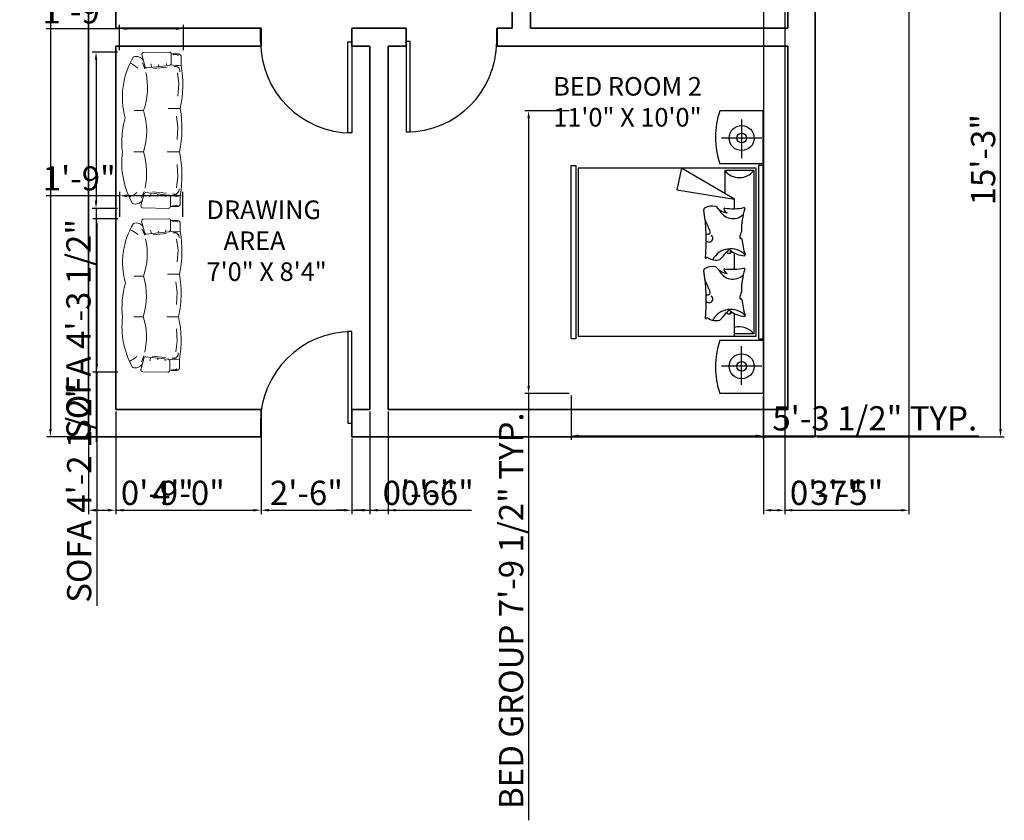
# Model space of a CAD drawing. Units: inches. Extents: x 3064 to 3427, y 2432 to 3115.
# Tile 1 of 3: x 3075 to 3401, y 2432 to 2696. Entities that reach past the tile are written whole.
import ezdxf

# ---------------------------------------------------------------- set-up
doc = ezdxf.new("R2010")
doc.units = ezdxf.units.IN
for name, color, linetype, lineweight in [('A-ANNO-DIMS', 2, 'Continuous', 13), ('A-AREA-IDEN', 7, 'Continuous', 18), ('A-DOOR', 4, 'Continuous', 25), ('A-WALL', 7, 'Continuous', 35), ('FUR', 42, 'Continuous', 18)]:
    doc.layers.add(name, color=color, linetype=linetype, lineweight=lineweight)
for name, color, linetype in [('HID', 11, 'Continuous'), ('SAN', 5, 'Continuous'), ('wood', 26, 'Continuous')]:
    doc.layers.add(name, color=color, linetype=linetype)
doc.styles.get("Standard").update_dxf_attribs({"font": 'arial.ttf'})
doc.dimstyles.new('ISO-25', dxfattribs={"dimtxt": 8, "dimasz": 2.5, "dimexe": 1.25, "dimexo": 0.625, "dimtad": 1, "dimdec": 0, "dimlunit": 4, "dimtxsty": 'Standard', "dimcen": 2.5, "dimadec": 0, "dimazin": 0, "dimtfac": 1, "dimtdec": 0, "dimtmove": 0, "dimatfit": 3, "dimfxl": 1, "dimarcsym": 0})

# ---------------------------------------------------------------- blocks, each defined once
blk = doc.blocks.new('A$C47AC156F')
at = {"layer": 'HID'}
for centre, radius, start, end in [((1.015, 1.799), 0.00933, 72.7248, 190.959), ((0.396, 1.679), 0.622, 352.7363, 10.959), ((1.25, 2.553), 0.781, 252.7248, 270.2702), ((0.966, 1.684), 0.155, 292.7628, 43.8922), ((1.385, 2.121), 0.373, 249.4168, 259.3085), ((1.317, 1.764), 0.00933, 259.3085, 10.689), ((1.336, 1.768), 0.00933, 96.2196, 190.689), ((1.25, 2.553), 0.781, 276.2196, 288.2114), ((1.645, 1.66), 0.21, 133.8947, 242.3952), ((1.258, 1.815), 0.249, 319.9211, 357.124), ((1.497, 1.803), 0.00933, 357.124, 108.2114), ((1.497, 1.803), 0.00933, 357.124, 108.2114), ((1.645, 1.799), 0.00933, 72.7248, 190.959), ((1.026, 1.679), 0.622, 352.7363, 10.959), ((1.88, 2.553), 0.781, 252.7248, 270.2702), ((1.596, 1.684), 0.155, 292.7628, 43.8922), ((2.015, 2.121), 0.373, 249.4168, 259.3085), ((1.947, 1.764), 0.00933, 259.3085, 10.689), ((1.966, 1.768), 0.00933, 96.2196, 190.689), ((1.88, 2.553), 0.781, 276.2196, 288.2114), ((2.275, 1.66), 0.21, 133.8947, 242.3952), ((1.888, 1.815), 0.249, 319.9211, 357.124), ((2.127, 1.803), 0.00933, 357.124, 108.2114), ((2.127, 1.803), 0.00933, 357.124, 108.2114), ((1.453, 1.646), 0.00933, 118.8315, 225.8329), ((2.727, 2.958), 1.838, 225.8329, 230.0245), ((0.994, -0.376), 2.088, 76.4982, 77.2888), ((1.445, 1.644), 0.0373, 312.662, 59.1573), ((2.083, 1.646), 0.00933, 118.8315, 225.8329), ((3.357, 2.958), 1.838, 225.8329, 230.0245), ((1.624, -0.376), 2.088, 76.4982, 77.2888), ((2.075, 1.644), 0.0373, 312.662, 59.1573), ((0.871, 1.658), 0.194, 311.6071, 349.7845), ((1.022, 1.599), 0.00933, 172.7363, 288.2985), ((1.005, 1.648), 0.0615, 288.2985, 335.7891), ((0.994, 3.644), 2.088, 282.7018, 282.7206), ((1.401, 1.508), 0.151, 327.1663, 15.7613), ((1.501, 1.658), 0.194, 311.6071, 349.7845), ((1.652, 1.599), 0.00933, 172.7363, 288.2985), ((1.635, 1.648), 0.0615, 288.2985, 335.7891), ((1.624, 3.644), 2.088, 282.7018, 282.7206), ((2.031, 1.508), 0.151, 327.1663, 15.7613), ((1.142, 1.469), 0.152, 167.3377, 211.666), ((1.012, 1.499), 0.0187, 131.6071, 167.3377), ((1.54, 0.631), 0.864, 109.049, 117.3823), ((1.264, 1.43), 0.0187, 2.6426, 109.049), ((1.326, 1.436), 0.0395, 312.3565, 145.7762), ((1.772, 1.469), 0.152, 167.3377, 211.666), ((1.642, 1.499), 0.0187, 131.6071, 167.3377), ((2.17, 0.631), 0.864, 109.049, 117.3823), ((1.894, 1.43), 0.0187, 2.6426, 109.049), ((1.956, 1.436), 0.0395, 312.3565, 145.7762), ((1.028, 1.399), 0.0187, 211.666, 279.4465), ((1.35, -0.534), 1.941, 84.5852, 99.4465), ((1.35, -0.534), 1.941, 96.386, 99.4465), ((1.132, 1.414), 0.0187, 276.386, 303.7955), ((1.301, 1.432), 0.0187, 182.6426, 192.7015), ((1.323, 1.437), 0.0414, 192.7015, 227.1556), ((1.543, 1.416), 0.0187, 147.1663, 264.3422), ((1.659, 1.399), 0.0187, 211.666, 279.4465), ((1.98, -0.534), 1.941, 84.5852, 99.4465), ((1.98, -0.534), 1.941, 96.386, 99.4465), ((1.762, 1.414), 0.0187, 276.386, 303.7955), ((1.931, 1.432), 0.0187, 182.6426, 192.7015), ((1.954, 1.437), 0.0414, 192.7015, 227.1556), ((2.173, 1.416), 0.0187, 147.1663, 264.3422)]:
    blk.add_arc(centre, radius, start, end, dxfattribs=at)
at = {"layer": 'SAN'}
for p, q in [((0.283, 1.985), (0.283, 1.566)), ((2.657, 1.985), (2.657, 1.566)), ((0.09, 1.775), (0.491, 1.775)), ((2.85, 1.775), (2.449, 1.775))]:
    blk.add_line(p, q, dxfattribs=at)
for centre, radius in [((0.283, 1.775), 0.13), ((2.657, 1.775), 0.13), ((0.283, 1.775), 0.05), ((2.657, 1.775), 0.05)]:
    blk.add_circle(centre, radius, dxfattribs=at)
at = {"layer": 'wood'}
for p, q in [((0, 1.998), (0, 1.548)), ((0.55, 1.998), (0, 1.998)), ((0.55, 1.998), (0.55, 1.548)), ((2.39, 1.998), (2.94, 1.998)), ((2.39, 1.998), (2.39, 1.548)), ((2.94, 1.998), (2.94, 1.548)), ((0.62, 1.9), (2.32, 1.9)), ((0.62, 1.9), (0.62, 1.6)), ((2.32, 1.9), (2.32, 1.7)), ((0.92, 1.7), (0.595, 1.15)), ((0.82, 1.1), (0.92, 1.7)), ((1.017, 1.7), (0.92, 1.7)), ((1.647, 1.7), (1.479, 1.7)), ((2.345, 1.7), (2.109, 1.7)), ((0.62, 1.6), (0.861, 1.6)), ((0.595, 1.15), (0.82, 1.1))]:
    blk.add_line(p, q, dxfattribs=at)
for points in [[(0.57, 1.95), (2.37, 1.95), (2.37, 2), (0.57, 2)], [(2.345, 0.075), (2.345, 1.925), (0.595, 1.925), (0.595, 0.075)], [(0.57, 0.05), (2.37, 0.05), (2.37, 0), (0.57, 0)]]:
    blk.add_lwpolyline(points, close=True, dxfattribs=at)
for centre, radius, start, end in [((0.504, 1.75), 0.19, 307.7826, 52.2174), ((2.436, 1.75), 0.19, 127.7826, 195.2747), ((0.275, 2.342), 0.84, 250.89, 289.11), ((2.665, 2.342), 0.84, 250.89, 289.11)]:
    blk.add_arc(centre, radius, start, end, dxfattribs=at)
blk = doc.blocks.new('3-s')
for p, q in [((-3104.73, -915.45), (-3104.73, -919.55)), ((-3099.98, -914.27), (-3099.98, -918.75)), ((-3086.85, -913.54), (-3099.1, -913.37)), ((-3087.27, -919.9), (-3085.85, -914.54)), ((-3098.98, -919.75), (-3088.27, -920.9)), ((-3091.42, -921.25), (-3098, -920.58)), ((-3097.59, -919.77), (-3097.73, -918.83)), ((-3093.97, -920.17), (-3094.1, -919.37)), ((-3090.75, -920.58), (-3090.21, -918.96)), ((-3086.18, -918.42), (-3087.39, -921.38)), ((-3102.96, -923.27), (-3103.63, -928.52)), ((-3103.63, -928.52), (-3103.23, -934.44)), ((-3104.33, -940.39), (-3098.51, -940.39)), ((-3087.08, -940.39), (-3082.49, -940.39)), ((-3103.63, -952.27), (-3103.23, -946.35)), ((-3102.96, -957.52), (-3103.63, -952.27)), ((-3104.73, -961.23), (-3098.92, -961.23)), ((-3087.15, -960.23), (-3082.56, -960.23)), ((-3104.04, -973.11), (-3103.63, -967.19)), ((-3103.37, -978.36), (-3104.04, -973.11)), ((-3091.82, -980.37), (-3098.4, -981.05)), ((-3098, -981.85), (-3098.13, -982.8)), ((-3094.37, -981.45), (-3094.51, -982.26)), ((-3091.15, -981.05), (-3090.61, -982.66)), ((-3086.59, -983.2), (-3087.79, -980.24)), ((-3105.14, -986.18), (-3105.14, -982.07))]:
    blk.add_line(p, q)
for points in [[(-3099.98, -914.27), (-3100.65, -914.23), (-3101.21, -914.21), (-3101.68, -914.19), (-3102.07, -914.18), (-3102.4, -914.18), (-3102.68, -914.19), (-3102.91, -914.21), (-3103.11, -914.22), (-3103.29, -914.24), (-3103.46, -914.26), (-3103.62, -914.29), (-3103.76, -914.33), (-3103.89, -914.36), (-3104.01, -914.41), (-3104.12, -914.47), (-3104.23, -914.53), (-3104.33, -914.6), (-3104.43, -914.69), (-3104.51, -914.78), (-3104.58, -914.89), (-3104.65, -915.01), (-3104.69, -915.14), (-3104.72, -915.29), (-3104.73, -915.45)], [(-3100.39, -987.35), (-3101.05, -987.39), (-3101.61, -987.42), (-3102.08, -987.43), (-3102.48, -987.44), (-3102.81, -987.44), (-3103.08, -987.43), (-3103.31, -987.42), (-3103.51, -987.4), (-3103.7, -987.38), (-3103.87, -987.36), (-3104.02, -987.33), (-3104.16, -987.3), (-3104.29, -987.26), (-3104.41, -987.21), (-3104.53, -987.16), (-3104.63, -987.09), (-3104.73, -987.02), (-3104.83, -986.94), (-3104.91, -986.84), (-3104.99, -986.73), (-3105.05, -986.61), (-3105.1, -986.48), (-3105.13, -986.34), (-3105.14, -986.18)]]:
    blk.add_lwpolyline(points)
blk.add_lwpolyline([(-3087.67, -981.72), (-3086.25, -987.09, -0.414214), (-3087.25, -988.09), (-3099.51, -988.25, -0.464301), (-3100.39, -987.35), (-3100.39, -982.87, -0.414214), (-3099.39, -981.87), (-3088.67, -980.72, -0.414214)], format="xyb", close=True)
for centre, radius, start, end in [((-3101.91, -917.78), 3.27, 72.9324, 119.1125), ((-3099.16, -914.2), 0.826, 85.8896, 185.5116), ((-3086.85, -914.54), 1, 0, 90), ((-3083.18, -919.47), 4.05, 71.0879, 146.7483), ((-3117.09, -935.46), 40.42, 352.9967, 29.3731), ((-3051.57, -928.95), 53.99, 169.9808, 192.2408), ((-3102.44, -907.13), 12.63, 259.551, 282.5683), ((-3101.95, -922.43), 2.24, 70.9224, 187.7848), ((-3098.98, -918.75), 1, 180, 270), ((-3088.27, -919.9), 1, 270, 0), ((-3074.56, -931.19), 13.81, 115.1439, 132.7066), ((-3055.23, -930.36), 33.39, 167.467, 197.4804), ((-3051.57, -951.84), 53.99, 167.7592, 190.0192), ((-3055.23, -950.42), 33.39, 162.5196, 197.0763), ((-3117.09, -945.32), 40.42, 343.5213, 7.0033), ((-3114.19, -966.81), 37.23, 329.0051, 15.6244), ((-3051.97, -972.68), 53.99, 167.7592, 190.0192), ((-3055.63, -971.26), 33.39, 160.7021, 192.533), ((-3102.84, -994.5), 12.63, 77.4317, 100.449), ((-3102.35, -979.2), 2.24, 172.2152, 289.0776), ((-3074.97, -970.43), 13.81, 227.2934, 244.8561), ((-3102.31, -983.84), 3.27, 240.8875, 287.0676), ((-3083.58, -982.16), 4.05, 213.2517, 288.9121)]:
    blk.add_arc(centre, radius, start, end)
blk = doc.blocks.new('*U12')
for p, q in [((-40, 0), (-40, 6)), ((0, 0), (0, 6))]:
    blk.add_line(p, q)
blk.add_lwpolyline([(0, 0), (0, -40), (-1.75, -40), (-1.75, 0)], close=True)
blk.add_arc((0, 0), 40, 180, 270)
blk = doc.blocks.new('*U13')
for p, q in [((0, 0), (0, 6)), ((40, 0), (40, 6))]:
    blk.add_line(p, q)
blk.add_lwpolyline([(0, 0), (0, -40), (1.75, -40), (1.75, 0)], close=True)
blk.add_arc((0, 0), 40, 270, 360)
blk = doc.blocks.new('*U11')
for p, q in [((0, 0), (0, -6)), ((-40, 0), (-40, -6))]:
    blk.add_line(p, q)
blk.add_lwpolyline([(0, 0), (0, 40), (-1.75, 40), (-1.75, 0)], close=True)
blk.add_arc((0, 0), 40, 90, 180)
blk = doc.blocks.new('*D16')
at = {"layer": 'A-ANNO-DIMS', "color": 0, "lineweight": -2, "transparency": 16777216}
for p, q in [((3097.42, 3014.45), (3084.25, 3014.45)), ((3085.5, 3011.95), (3085.5, 2560.95)), ((3097.42, 2558.45), (3084.25, 2558.45))]:
    blk.add_line(p, q, dxfattribs=at)
at = {"layer": 'A-ANNO-DIMS', "color": 0, "transparency": 16777216}
for points in [[(3085.09, 3011.95), (3085.92, 3011.95), (3085.5, 3014.45)], [(3085.09, 2560.95), (3085.92, 2560.95), (3085.5, 2558.45)]]:
    blk.add_solid(points, dxfattribs=at)
at = {"layer": 'Defpoints', "color": 0, "transparency": 16777216}
for p in [(3098.05, 3014.45), (3085.5, 2558.45), (3098.05, 2558.45)]:
    blk.add_point(p, dxfattribs=at)
at = {"layer": 'A-ANNO-DIMS', "color": 0, "transparency": 16777216, "insert": (3080.79, 2786.45), "char_height": 8, "attachment_point": 5, "rotation": 90}
blk.add_mtext("38'", dxfattribs=at)
blk = doc.blocks.new('*D18')
at = {"layer": 'A-ANNO-DIMS', "color": 0, "lineweight": -2, "transparency": 16777216}
for p, q in [((3256.83, 2666.09), (3242.2, 2666.09)), ((3243.45, 2663.59), (3243.45, 2575.23)), ((3256.83, 2572.73), (3242.2, 2572.73)), ((3243.45, 2572.73), (3243.45, 2431.75))]:
    blk.add_line(p, q, dxfattribs=at)
at = {"layer": 'A-ANNO-DIMS', "color": 0, "transparency": 16777216}
for points in [[(3243.03, 2663.59), (3243.87, 2663.59), (3243.45, 2666.09)], [(3243.03, 2575.23), (3243.87, 2575.23), (3243.45, 2572.73)]]:
    blk.add_solid(points, dxfattribs=at)
at = {"layer": 'Defpoints', "color": 0, "transparency": 16777216}
for p in [(3257.45, 2666.09), (3243.45, 2572.73), (3257.45, 2572.73)]:
    blk.add_point(p, dxfattribs=at)
at = {"layer": 'A-ANNO-DIMS', "color": 0, "transparency": 16777216, "insert": (3238.69, 2500.99), "char_height": 8, "attachment_point": 5, "rotation": 90}
blk.add_mtext('BED GROUP 7\'-9 1/2" TYP.', dxfattribs=at)
blk = doc.blocks.new('*D19')
at = {"layer": 'A-ANNO-DIMS', "color": 0, "lineweight": -2, "transparency": 16777216}
for p, q in [((3257.45, 2572.1), (3257.45, 2557.47)), ((3320.97, 2572.1), (3320.97, 2557.47)), ((3259.95, 2558.72), (3318.47, 2558.72)), ((3320.97, 2558.72), (3392.12, 2558.72))]:
    blk.add_line(p, q, dxfattribs=at)
at = {"layer": 'A-ANNO-DIMS', "color": 0, "transparency": 16777216}
for points in [[(3259.95, 2559.14), (3259.95, 2558.3), (3257.45, 2558.72)], [(3318.47, 2559.14), (3318.47, 2558.3), (3320.97, 2558.72)]]:
    blk.add_solid(points, dxfattribs=at)
at = {"layer": 'Defpoints', "color": 0, "transparency": 16777216}
for p in [(3257.45, 2572.73), (3320.97, 2572.73), (3320.97, 2558.72)]:
    blk.add_point(p, dxfattribs=at)
at = {"layer": 'A-ANNO-DIMS', "color": 0, "transparency": 16777216, "insert": (3357.79, 2563.49), "char_height": 8, "attachment_point": 5}
blk.add_mtext('5\'-3 1/2" TYP.', dxfattribs=at)
blk = doc.blocks.new('*D20')
at = {"layer": 'A-ANNO-DIMS', "color": 0, "lineweight": -2, "transparency": 16777216}
for p, q in [((3107.75, 2630.44), (3099.53, 2630.44)), ((3100.78, 2627.94), (3100.78, 2582.27)), ((3107.75, 2579.77), (3099.53, 2579.77)), ((3100.78, 2579.77), (3100.78, 2502.62))]:
    blk.add_line(p, q, dxfattribs=at)
at = {"layer": 'A-ANNO-DIMS', "color": 0, "transparency": 16777216}
for points in [[(3100.36, 2627.94), (3101.2, 2627.94), (3100.78, 2630.44)], [(3100.36, 2582.27), (3101.2, 2582.27), (3100.78, 2579.77)]]:
    blk.add_solid(points, dxfattribs=at)
at = {"layer": 'Defpoints', "color": 0, "transparency": 16777216}
for p in [(3108.38, 2630.44), (3100.78, 2579.77), (3108.38, 2579.77)]:
    blk.add_point(p, dxfattribs=at)
at = {"layer": 'A-ANNO-DIMS', "color": 0, "transparency": 16777216, "insert": (3096.01, 2539.94), "char_height": 8, "attachment_point": 5, "rotation": 90}
blk.add_mtext('SOFA 4\'-2 1/2"', dxfattribs=at)
blk = doc.blocks.new('*D21')
at = {"layer": 'A-ANNO-DIMS', "color": 0, "lineweight": -2, "transparency": 16777216}
for p, q in [((3108.38, 2638.04), (3084.12, 2638.04)), ((3108.38, 2631.07), (3108.38, 2639.29)), ((3126.7, 2638.04), (3110.88, 2638.04)), ((3129.2, 2631.07), (3129.2, 2639.29))]:
    blk.add_line(p, q, dxfattribs=at)
at = {"layer": 'A-ANNO-DIMS', "color": 0, "transparency": 16777216}
for points in [[(3110.88, 2638.46), (3110.88, 2637.62), (3108.38, 2638.04)], [(3126.7, 2638.46), (3126.7, 2637.62), (3129.2, 2638.04)]]:
    blk.add_solid(points, dxfattribs=at)
at = {"layer": 'Defpoints', "color": 0, "transparency": 16777216}
for p in [(3108.38, 2638.04), (3108.38, 2630.44), (3129.2, 2630.44)]:
    blk.add_point(p, dxfattribs=at)
at = {"layer": 'A-ANNO-DIMS', "color": 0, "transparency": 16777216, "insert": (3095, 2642.75), "char_height": 8, "attachment_point": 5}
blk.add_mtext('1\'-9"', dxfattribs=at)
blk = doc.blocks.new('*D22')
at = {"layer": 'A-ANNO-DIMS', "color": 0, "lineweight": -2, "transparency": 16777216}
for p, q in [((3107.67, 2685.48), (3099.3, 2685.48)), ((3100.55, 2682.98), (3100.55, 2636.37)), ((3107.67, 2633.87), (3099.3, 2633.87)), ((3100.55, 2633.87), (3100.55, 2556.72))]:
    blk.add_line(p, q, dxfattribs=at)
at = {"layer": 'A-ANNO-DIMS', "color": 0, "transparency": 16777216}
for points in [[(3100.14, 2682.98), (3100.97, 2682.98), (3100.55, 2685.48)], [(3100.14, 2636.37), (3100.97, 2636.37), (3100.55, 2633.87)]]:
    blk.add_solid(points, dxfattribs=at)
at = {"layer": 'Defpoints', "color": 0, "transparency": 16777216}
for p in [(3108.3, 2685.48), (3100.55, 2633.87), (3108.3, 2633.87)]:
    blk.add_point(p, dxfattribs=at)
at = {"layer": 'A-ANNO-DIMS', "color": 0, "transparency": 16777216, "insert": (3095.79, 2594.05), "char_height": 8, "attachment_point": 5, "rotation": 90}
blk.add_mtext('SOFA 4\'-3 1/2"', dxfattribs=at)
blk = doc.blocks.new('*D23')
at = {"layer": 'A-ANNO-DIMS', "color": 0, "lineweight": -2, "transparency": 16777216}
for p, q in [((3108.3, 2693.22), (3084.03, 2693.22)), ((3108.3, 2686.11), (3108.3, 2694.47)), ((3127, 2693.22), (3110.8, 2693.22)), ((3129.5, 2686.11), (3129.5, 2694.47))]:
    blk.add_line(p, q, dxfattribs=at)
at = {"layer": 'A-ANNO-DIMS', "color": 0, "transparency": 16777216}
for points in [[(3110.8, 2693.64), (3110.8, 2692.81), (3108.3, 2693.22)], [(3127, 2693.64), (3127, 2692.81), (3129.5, 2693.22)]]:
    blk.add_solid(points, dxfattribs=at)
at = {"layer": 'Defpoints', "color": 0, "transparency": 16777216}
for p in [(3108.3, 2693.22), (3108.3, 2685.48), (3129.5, 2685.48)]:
    blk.add_point(p, dxfattribs=at)
at = {"layer": 'A-ANNO-DIMS', "color": 0, "transparency": 16777216, "insert": (3094.91, 2697.93), "char_height": 8, "attachment_point": 5}
blk.add_mtext('1\'-9"', dxfattribs=at)
blk = doc.blocks.new('*D31')
at = {"layer": 'A-ANNO-DIMS', "color": 0, "lineweight": -2, "transparency": 16777216}
for p, q in [((3107.05, 2566.83), (3107.05, 2532.92)), ((3098.05, 2557.83), (3098.05, 2532.92)), ((3100.55, 2534.17), (3104.55, 2534.17)), ((3107.05, 2534.17), (3132.06, 2534.17))]:
    blk.add_line(p, q, dxfattribs=at)
at = {"layer": 'A-ANNO-DIMS', "color": 0, "transparency": 16777216}
for points in [[(3100.55, 2534.59), (3100.55, 2533.75), (3098.05, 2534.17)], [(3104.55, 2534.59), (3104.55, 2533.75), (3107.05, 2534.17)]]:
    blk.add_solid(points, dxfattribs=at)
at = {"layer": 'Defpoints', "color": 0, "transparency": 16777216}
for p in [(3107.05, 2567.45), (3098.05, 2558.45), (3107.05, 2534.17)]:
    blk.add_point(p, dxfattribs=at)
at = {"layer": 'A-ANNO-DIMS', "color": 0, "transparency": 16777216, "insert": (3120.8, 2538.88), "char_height": 8, "attachment_point": 5}
blk.add_mtext('0\'-9"', dxfattribs=at)
blk = doc.blocks.new('*D32')
at = {"layer": 'A-ANNO-DIMS', "color": 0, "lineweight": -2, "transparency": 16777216}
for p, q in [((3107.05, 2566.83), (3107.05, 2532.92)), ((3155.05, 2566.83), (3155.05, 2532.92)), ((3109.55, 2534.17), (3152.55, 2534.17))]:
    blk.add_line(p, q, dxfattribs=at)
at = {"layer": 'A-ANNO-DIMS', "color": 0, "transparency": 16777216}
for points in [[(3109.55, 2534.59), (3109.55, 2533.75), (3107.05, 2534.17)], [(3152.55, 2534.59), (3152.55, 2533.75), (3155.05, 2534.17)]]:
    blk.add_solid(points, dxfattribs=at)
at = {"layer": 'Defpoints', "color": 0, "transparency": 16777216}
for p in [(3107.05, 2567.45), (3155.05, 2567.45), (3155.05, 2534.17)]:
    blk.add_point(p, dxfattribs=at)
at = {"layer": 'A-ANNO-DIMS', "color": 0, "transparency": 16777216, "insert": (3131.05, 2538.88), "char_height": 8, "attachment_point": 5}
blk.add_mtext('4\'-0"', dxfattribs=at)
blk = doc.blocks.new('*D33')
at = {"layer": 'A-ANNO-DIMS', "color": 0, "lineweight": -2, "transparency": 16777216}
for p, q in [((3155.05, 2557.83), (3155.05, 2532.92)), ((3185.05, 2557.83), (3185.05, 2532.92)), ((3157.55, 2534.17), (3182.55, 2534.17))]:
    blk.add_line(p, q, dxfattribs=at)
at = {"layer": 'A-ANNO-DIMS', "color": 0, "transparency": 16777216}
for points in [[(3157.55, 2534.59), (3157.55, 2533.75), (3155.05, 2534.17)], [(3182.55, 2534.59), (3182.55, 2533.75), (3185.05, 2534.17)]]:
    blk.add_solid(points, dxfattribs=at)
at = {"layer": 'Defpoints', "color": 0, "transparency": 16777216}
for p in [(3155.05, 2558.45), (3185.05, 2558.45), (3185.05, 2534.17)]:
    blk.add_point(p, dxfattribs=at)
at = {"layer": 'A-ANNO-DIMS', "color": 0, "transparency": 16777216, "insert": (3170.05, 2538.88), "char_height": 8, "attachment_point": 5}
blk.add_mtext('2\'-6"', dxfattribs=at)
blk = doc.blocks.new('*D34')
at = {"layer": 'A-ANNO-DIMS', "color": 0, "lineweight": -2, "transparency": 16777216}
for p, q in [((3191.05, 2566.83), (3191.05, 2532.92)), ((3197.05, 2566.83), (3197.05, 2532.92)), ((3188.55, 2534.17), (3186.05, 2534.17)), ((3191.05, 2534.17), (3197.05, 2534.17)), ((3199.55, 2534.17), (3224.56, 2534.17))]:
    blk.add_line(p, q, dxfattribs=at)
at = {"layer": 'A-ANNO-DIMS', "color": 0, "transparency": 16777216}
for points in [[(3188.55, 2534.59), (3188.55, 2533.75), (3191.05, 2534.17)], [(3199.55, 2534.59), (3199.55, 2533.75), (3197.05, 2534.17)]]:
    blk.add_solid(points, dxfattribs=at)
at = {"layer": 'Defpoints', "color": 0, "transparency": 16777216}
for p in [(3191.05, 2567.45), (3197.05, 2567.45), (3197.05, 2534.17)]:
    blk.add_point(p, dxfattribs=at)
at = {"layer": 'A-ANNO-DIMS', "color": 0, "transparency": 16777216, "insert": (3213.3, 2538.88), "char_height": 8, "attachment_point": 5}
blk.add_mtext('0\'-6"', dxfattribs=at)
blk = doc.blocks.new('*D35')
at = {"layer": 'A-ANNO-DIMS', "color": 0, "lineweight": -2, "transparency": 16777216}
for p, q in [((3191.05, 2566.83), (3191.05, 2532.92)), ((3185.05, 2557.83), (3185.05, 2532.92)), ((3182.55, 2534.17), (3180.05, 2534.17)), ((3185.05, 2534.17), (3191.05, 2534.17)), ((3193.55, 2534.17), (3218.56, 2534.17))]:
    blk.add_line(p, q, dxfattribs=at)
at = {"layer": 'A-ANNO-DIMS', "color": 0, "transparency": 16777216}
for points in [[(3182.55, 2534.59), (3182.55, 2533.75), (3185.05, 2534.17)], [(3193.55, 2534.59), (3193.55, 2533.75), (3191.05, 2534.17)]]:
    blk.add_solid(points, dxfattribs=at)
at = {"layer": 'Defpoints', "color": 0, "transparency": 16777216}
for p in [(3191.05, 2567.45), (3185.05, 2558.45), (3191.05, 2534.17)]:
    blk.add_point(p, dxfattribs=at)
at = {"layer": 'A-ANNO-DIMS', "color": 0, "transparency": 16777216, "insert": (3207.3, 2538.88), "char_height": 8, "attachment_point": 5}
blk.add_mtext('0\'-6"', dxfattribs=at)
blk = doc.blocks.new('*D36')
at = {"layer": 'A-ANNO-DIMS', "color": 0, "lineweight": -2, "transparency": 16777216}
for p, q in [((3375.67, 2741.45), (3400.58, 2741.45)), ((3399.33, 2560.95), (3399.33, 2738.95)), ((3338.67, 2558.45), (3400.58, 2558.45))]:
    blk.add_line(p, q, dxfattribs=at)
at = {"layer": 'A-ANNO-DIMS', "color": 0, "transparency": 16777216}
for points in [[(3398.91, 2738.95), (3399.74, 2738.95), (3399.33, 2741.45)], [(3398.91, 2560.95), (3399.74, 2560.95), (3399.33, 2558.45)]]:
    blk.add_solid(points, dxfattribs=at)
at = {"layer": 'Defpoints', "color": 0, "transparency": 16777216}
for p in [(3375.05, 2741.45), (3399.33, 2741.45), (3338.05, 2558.45)]:
    blk.add_point(p, dxfattribs=at)
at = {"layer": 'A-ANNO-DIMS', "color": 0, "transparency": 16777216, "insert": (3394.61, 2649.95), "char_height": 8, "attachment_point": 5, "rotation": 90}
blk.add_mtext('15\'-3"', dxfattribs=at)
blk = doc.blocks.new('*D37')
at = {"layer": 'A-ANNO-DIMS', "color": 0, "lineweight": -2, "transparency": 16777216}
for p, q in [((3328.05, 2746.83), (3328.05, 2532.92)), ((3369.05, 2746.83), (3369.05, 2532.92)), ((3330.55, 2534.17), (3366.55, 2534.17))]:
    blk.add_line(p, q, dxfattribs=at)
at = {"layer": 'A-ANNO-DIMS', "color": 0, "transparency": 16777216}
for points in [[(3330.55, 2534.59), (3330.55, 2533.75), (3328.05, 2534.17)], [(3366.55, 2534.59), (3366.55, 2533.75), (3369.05, 2534.17)]]:
    blk.add_solid(points, dxfattribs=at)
at = {"layer": 'Defpoints', "color": 0, "transparency": 16777216}
for p in [(3328.05, 2747.45), (3369.05, 2747.45), (3369.05, 2534.17)]:
    blk.add_point(p, dxfattribs=at)
at = {"layer": 'A-ANNO-DIMS', "color": 0, "transparency": 16777216, "insert": (3348.55, 2538.88), "char_height": 8, "attachment_point": 5}
blk.add_mtext('3\'-5"', dxfattribs=at)
blk = doc.blocks.new('*D38')
at = {"layer": 'A-ANNO-DIMS', "color": 0, "lineweight": -2, "transparency": 16777216}
for p, q in [((3321.05, 2746.83), (3321.05, 2532.92)), ((3328.05, 2746.83), (3328.05, 2532.92)), ((3323.55, 2534.17), (3325.55, 2534.17)), ((3328.05, 2534.17), (3353.06, 2534.17))]:
    blk.add_line(p, q, dxfattribs=at)
at = {"layer": 'A-ANNO-DIMS', "color": 0, "transparency": 16777216}
for points in [[(3323.55, 2534.59), (3323.55, 2533.75), (3321.05, 2534.17)], [(3325.55, 2534.59), (3325.55, 2533.75), (3328.05, 2534.17)]]:
    blk.add_solid(points, dxfattribs=at)
at = {"layer": 'Defpoints', "color": 0, "transparency": 16777216}
for p in [(3321.05, 2747.45), (3328.05, 2747.45), (3328.05, 2534.17)]:
    blk.add_point(p, dxfattribs=at)
at = {"layer": 'A-ANNO-DIMS', "color": 0, "transparency": 16777216, "insert": (3341.8, 2538.88), "char_height": 8, "attachment_point": 5}
blk.add_mtext('0\'-7"', dxfattribs=at)

msp = doc.modelspace()

# ---------------------------------------------------------------- linework, layer by layer
at = {"layer": 'A-WALL'}
for p, q in [((3098.05, 2558.45), (3098.05, 3014.45)), ((3107.05, 2693.45), (3107.05, 2882.45)), ((3329.05, 2741.45), (3329.05, 2693.45)), ((3338.05, 2741.45), (3338.05, 2558.45)), ((3238.05, 2693.45), (3238.05, 2699.45)), ((3244.05, 2693.45), (3244.05, 2699.45)), ((3107.05, 2693.45), (3155.05, 2693.45)), ((3155.05, 2687.45), (3155.05, 2693.45)), ((3185.05, 2693.45), (3203.05, 2693.45)), ((3185.05, 2687.45), (3185.05, 2693.45)), ((3203.05, 2687.45), (3203.05, 2693.45)), ((3233.05, 2693.45), (3238.05, 2693.45)), ((3233.05, 2687.45), (3233.05, 2693.45)), ((3244.05, 2693.45), (3329.05, 2693.45)), ((3107.05, 2567.45), (3107.05, 2687.45)), ((3107.05, 2687.45), (3155.05, 2687.45)), ((3185.05, 2687.45), (3191.05, 2687.45)), ((3191.05, 2567.45), (3191.05, 2687.45)), ((3197.05, 2567.45), (3197.05, 2687.45)), ((3197.05, 2687.45), (3203.05, 2687.45)), ((3233.05, 2687.45), (3329.05, 2687.45)), ((3329.05, 2687.45), (3329.05, 2567.45)), ((3155.05, 2567.45), (3107.05, 2567.45)), ((3155.05, 2558.45), (3155.05, 2567.45)), ((3185.05, 2558.45), (3185.05, 2567.45)), ((3191.05, 2567.45), (3185.05, 2567.45)), ((3329.05, 2567.45), (3197.05, 2567.45)), ((3155.05, 2558.45), (3098.05, 2558.45)), ((3338.05, 2558.45), (3185.05, 2558.45))]:
    msp.add_line(p, q, dxfattribs=at)

# ---------------------------------------------------------------- block references
at = {"layer": 'A-DOOR'}
for name, p, xscale, yscale, zscale in [('*U12', (3185.05, 2688.93), 0.7530531738866394, 0.7530531738866394, 0.7530531738866394), ('*U13', (3203.05, 2688.97), 0.7465626960772728, 0.7465626960772728, 0.7465626960772728), ('*U11', (3185.05, 2562.98), 0.7546152823496514, 0.7546152823496514, 0.7546152823496514)]:
    msp.add_blockref(name, p, dxfattribs=dict(at, xscale=xscale, yscale=yscale, zscale=zscale))
at = {"layer": 'FUR'}
for name, p, xscale, yscale, zscale, rotation in [('3-s', (989.55, 2004.67), 0.6888939635839342, 0.6888939635839342, 0.6888939635839342, 180), ('A$C47AC156F', (3257.45, 2666.09), 31.75566245105898, 31.75566245105898, 31.75566245105898, 270.0000000000002), ('3-s', (1028.21, 1962.02, 14.04), 0.6763533658241933, 0.6763533658241933, 0.6763533658241933, 180)]:
    msp.add_blockref(name, p, dxfattribs=dict(at, xscale=xscale, yscale=yscale, zscale=zscale, rotation=rotation))

# ---------------------------------------------------------------- texts
at = {"layer": 'A-AREA-IDEN', "char_height": 6.1325, "attachment_point": 1}
for s, insert in [('BED ROOM 2\\P11\'0" X 10\'0"', (3251.59, 2677.25)), ('DRAWING\\P   AREA\\P7\'0" X 8\'4"', (3137.07, 2636.48))]:
    msp.add_mtext_dynamic_manual_height_columns(s, width=649.6086, gutter_width=30.66, heights=[0], dxfattribs=dict(at, insert=insert))

# ---------------------------------------------------------------- dimensions: what is measured, and where the dimension line sits
at = {"layer": 'A-ANNO-DIMS'}
for base, p1, p2, angle, override, picture, middle in [((3085.5, 2558.45), (3098.05, 3014.45), (3098.05, 2558.45), 90, {"dimclrd": 0, "dimclre": 0, "dimclrt": 0}, '*D16', (3080.79, 2786.45)), ((3399.33, 2741.45), (3338.05, 2558.45), (3375.05, 2741.45), 90, {"dimdec": 1, "dimlfac": 1, "dimrnd": 0, "dimzin": 1, "dimdsep": 46, "dimlunit": 4, "dimfrac": 2}, '*D36', (3394.61, 2649.95)), ((3108.3, 2693.22), (3129.5, 2685.48), (3108.3, 2685.48), 180, {"dimdec": 1, "dimlfac": 1, "dimrnd": 0, "dimzin": 1, "dimdsep": 46, "dimlunit": 4, "dimfrac": 2}, '*D23', (3094.91, 2697.93)), ((3108.38, 2638.04), (3129.2, 2630.44), (3108.38, 2630.44), 180, {"dimdec": 1, "dimlfac": 1, "dimrnd": 0, "dimzin": 1, "dimdsep": 46, "dimlunit": 4, "dimfrac": 2}, '*D21', (3095, 2642.75))]:
    dim = msp.add_linear_dim(base=base, p1=p1, p2=p2, angle=angle, dimstyle='ISO-25', override=override, dxfattribs=at)
    dim.commit()
    dim.dimension.update_dxf_attribs({"geometry": picture, "text_midpoint": middle})
for base, p1, p2, picture, middle in [((3328.05, 2534.17), (3321.05, 2747.45), (3328.05, 2747.45), '*D38', (3341.8, 2538.88)), ((3369.05, 2534.17), (3328.05, 2747.45), (3369.05, 2747.45), '*D37', (3348.55, 2538.88)), ((3107.05, 2534.17), (3098.05, 2558.45), (3107.05, 2567.45), '*D31', (3120.8, 2538.88)), ((3155.05, 2534.17), (3107.05, 2567.45), (3155.05, 2567.45), '*D32', (3131.05, 2538.88)), ((3191.05, 2534.17), (3185.05, 2558.45), (3191.05, 2567.45), '*D35', (3207.3, 2538.88)), ((3197.05, 2534.17), (3191.05, 2567.45), (3197.05, 2567.45), '*D34', (3213.3, 2538.88)), ((3185.05, 2534.17), (3155.05, 2558.45), (3185.05, 2558.45), '*D33', (3170.05, 2538.88))]:
    dim = msp.add_linear_dim(base=base, p1=p1, p2=p2, dimstyle='ISO-25', override={"dimdec": 1, "dimlfac": 1, "dimrnd": 0, "dimzin": 1, "dimdsep": 46, "dimlunit": 4, "dimfrac": 2}, dxfattribs=at)
    dim.commit()
    dim.dimension.update_dxf_attribs({"geometry": picture, "text_midpoint": middle})
for base, p1, p2, text, picture, middle in [((3100.55, 2633.87), (3108.3, 2685.48), (3108.3, 2633.87), 'SOFA <>', '*D22', (3095.79, 2594.05)), ((3243.45, 2572.73), (3257.45, 2666.09), (3257.45, 2572.73), 'BED GROUP <> TYP.', '*D18', (3238.69, 2500.99)), ((3100.78, 2579.77), (3108.38, 2630.44), (3108.38, 2579.77), 'SOFA <>', '*D20', (3096.01, 2539.94))]:
    dim = msp.add_linear_dim(base=base, p1=p1, p2=p2, angle=270, text=text, dimstyle='ISO-25', override={"dimdec": 1, "dimlfac": 1, "dimrnd": 0, "dimzin": 1, "dimdsep": 46, "dimlunit": 4, "dimfrac": 2}, dxfattribs=at)
    dim.commit()
    dim.dimension.update_dxf_attribs({"geometry": picture, "text_midpoint": middle})
dim = msp.add_linear_dim(base=(3320.97, 2558.72), p1=(3257.45, 2572.73), p2=(3320.97, 2572.73), text='<> TYP.', dimstyle='ISO-25', override={"dimdec": 1, "dimlfac": 1, "dimrnd": 0, "dimzin": 1, "dimdsep": 46, "dimlunit": 4, "dimfrac": 2}, dxfattribs=at)
dim.commit()
dim.dimension.update_dxf_attribs({"geometry": '*D19', "text_midpoint": (3357.79, 2563.49)})

doc.saveas('drawing.dxf')
